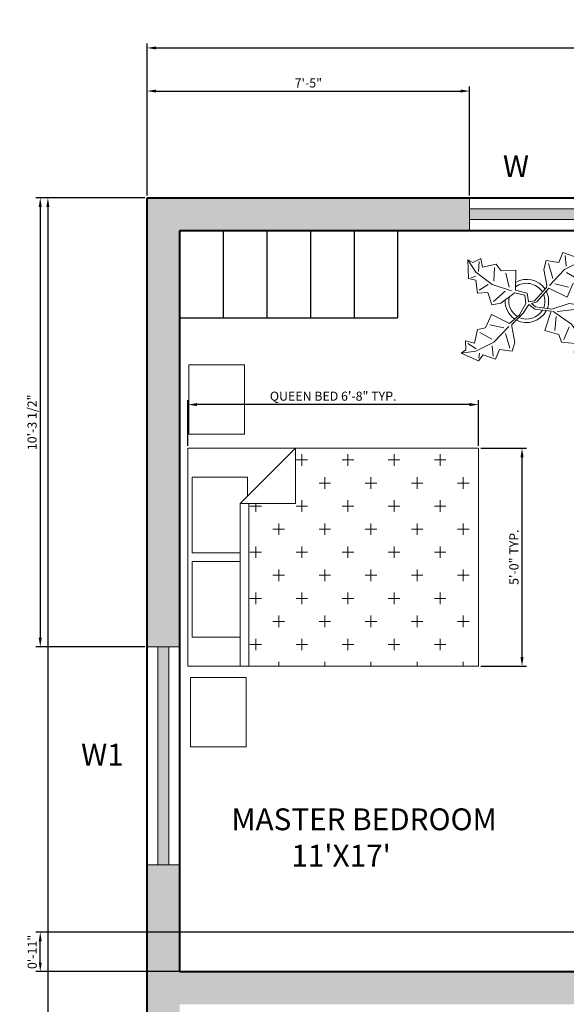
# Model space of a CAD drawing. Units: inches. Extents: x 4432 to 4859, y 8121 to 8698.
# Tile 3 of 4: x 4432 to 4583, y 8410 to 8681. Entities that reach past the tile are written whole.
import ezdxf

# ---------------------------------------------------------------- set-up
doc = ezdxf.new("R2010")
doc.units = ezdxf.units.IN
for name, color, linetype, lineweight in [('A-ANNO-DIMS', 2, 'Continuous', 18), ('A-ANNO-TEXT', 7, 'Continuous', 18), ('A-AREA-IDEN', 4, 'Continuous', 18), ('A-FLOR-CASE', 8, 'Continuous', 25), ('A-FURN', 8, 'Continuous', 18), ('A-FURN-PATT', 8, 'Continuous', 13), ('A-FURN-PLNT', 94, 'Continuous', 13), ('A-GLAZ', 4, 'Continuous', 20), ('A-GLAZ-PATT', 4, 'Continuous', 13), ('A-WALL', 7, 'Continuous', 40)]:
    doc.layers.add(name, color=color, linetype=linetype, lineweight=lineweight)
doc.layers.add('A-WALL-PATT', color=219, linetype='Continuous', lineweight=13, true_color=0x642165)
doc.styles.get("Standard").update_dxf_attribs({"font": 'arial.ttf'})
doc.dimstyles.new('ISO-25', dxfattribs={"dimtxt": 2.5, "dimasz": 2.5, "dimexe": 1.25, "dimexo": 0.625, "dimtad": 1, "dimlunit": 3, "dimtxsty": 'Standard', "dimcen": 2.5, "dimadec": 0, "dimazin": 0, "dimtfac": 1, "dimtmove": 0, "dimatfit": 3, "dimfxl": 1, "dimarcsym": 0})

# ---------------------------------------------------------------- blocks, each defined once
blk = doc.blocks.new('Bed - Queen')
for p, q in [((0, -80.00003), (0, 0)), ((0, 0), (59.99999, 0)), ((59.99999, 0), (59.99999, -80.00003)), ((7.99999, -1.2), (28.79998, -1.2)), ((7.99999, -14.4), (7.99999, -1.2)), ((28.79998, -1.2), (28.79998, -14.4)), ((31.19999, -1.2), (51.99999, -1.2)), ((31.19999, -14.4), (31.19999, -1.2)), ((51.99999, -1.2), (51.99999, -16.4)), ((0, -14.4), (44.8, -14.4)), ((59.99999, -29.6), (44.8, -14.4)), ((44.8, -14.4), (44.8, -29.6)), ((44.8, -16.8), (0, -16.8)), ((51.99999, -16.4), (46.79936, -16.4)), ((44.8, -29.6), (59.99999, -29.6)), ((59.99999, -80.00003), (0, -80.00003))]:
    blk.add_line(p, q)
blk = doc.blocks.new('Plant - Rubber or Philodendron')
for p, q in [((13.3837, 12.301), (14.68, 13.9039)), ((14.68, 13.9039), (19.3848, 11.8146)), ((-16.2005, 11.4774), (-13.9899, 8.1064)), ((-16.2005, 11.4774), (-14.8639, 10.7964)), ((-16.0159, 6.3329), (-16.2005, 11.4774)), ((-14.8639, 10.7964), (-12.6195, 11.8975)), ((-13.3174, 8.325), (-13.0735, 11.0065)), ((-12.6195, 11.8975), (-12.1909, 9.4345)), ((4.6914, 8.8812), (5.3859, 11.2828)), ((5.3859, 11.2828), (8.8871, 10.7908)), ((8.8871, 10.7908), (9.9809, 13.4933)), ((9.9809, 13.4933), (13.3837, 12.301)), ((15.3859, 11.3055), (10.3916, 8.7942)), ((10.5828, 12.6946), (10.8893, 9.7953)), ((14.5816, 13.2037), (14.3848, 11.8033)), ((19.3848, 11.8146), (15.3859, 11.3055)), ((19.3848, 11.8146), (18.1868, 10.9119)), ((18.1868, 10.9119), (18.1925, 8.4119)), ((-12.1909, 9.4345), (-8.3829, 10.3)), ((-8.8369, 9.409), (-9.0894, 5.6095)), ((-8.3829, 10.3), (-7.0549, 8.501)), ((-7.0549, 8.501), (-3.0284, 8.6941)), ((-3.0284, 8.6941), (-3.0709, 3.1041)), ((4.6914, 8.8812), (5.5014, 4.4831)), ((5.9878, 10.4842), (7.1971, 6.3869)), ((10.3916, 8.7942), (6.2847, 4.4028)), ((15.7909, 9.1065), (14.8995, 5.3044)), ((15.2875, 10.6053), (17.5907, 9.2105)), ((18.1925, 8.4119), (15.7909, 9.1065)), ((-14.0069, 5.8704), (-16.0159, 6.3329)), ((-15.3434, 6.5514), (-13.9984, 6.9884)), ((-13.5868, 2.2894), (-14.0069, 5.8704)), ((-13.9899, 8.1064), (-9.5434, 4.7185)), ((-4.8529, 4.012), (-5.7184, 7.82)), ((14.2977, 6.1031), (10.9934, 7.9956)), ((-13.1329, 3.1804), (-10.6614, 4.727)), ((-9.5434, 4.7185), (-4.1917, 2.9888)), ((-9.1318, 0.0195), (-5.9793, 2.9025)), ((-3.0709, 3.1041), (0.0797, 2.3163)), ((2.1141, 0.2298), (5.4346, 3.9146)), ((6.1032, 3.6844), (2.8262, -0.031)), ((5.4346, 3.9146), (5.5014, 4.4831)), ((11.1089, 1.1958), (6.1032, 3.6844)), ((7.7005, 4.8881), (11.5025, 3.9967)), ((12.7005, 4.8994), (11.1089, 1.1958)), ((14.8995, 5.3044), (12.7005, 4.8994)), ((-10.6784, 2.491), (-13.5868, 2.2894)), ((-9.5858, -0.8715), (-10.6784, 2.491)), ((-7.1228, -0.443), (-3.5248, 2.2131)), ((-3.5248, 2.2131), (-3.3011, 2.4355)), ((-3.3011, 2.4355), (-0.5306, 1.7947)), ((-0.5306, 1.7947), (-0.2255, -0.5527)), ((-0.5306, 1.7947), (-0.5306, 1.7947)), ((0.0797, 2.3163), (0.4866, -0.031)), ((0.4866, -0.031), (2.1141, 0.2298)), ((-7.1228, -0.443), (-9.5858, -0.8715)), ((-2.019, -3.6148), (-0.2255, -0.5527)), ((-0.9375, -3.1608), (0.5883, -0.8135)), ((0.5883, -0.8135), (2.2447, -2.0916)), ((2.8262, -0.031), (1.3003, -0.5527)), ((1.3003, -0.5527), (2.4193, -1.4655)), ((2.2447, -2.0916), (6.7108, -2.6626)), ((2.4193, -1.4655), (6.895, -2.1175)), ((4.943, -7.9659), (6.7108, -2.6626)), ((11.6605, -0.5413), (6.895, -2.1175)), ((12.3677, -6.1981), (7.219, -2.6772)), ((8.3544, -2.7453), (13.1973, -2.1704)), ((11.6605, -0.5413), (14.1354, -0.8948)), ((14.1354, -0.8948), (14.1354, -4.4304)), ((-11.3237, -7.2629), (-9.7321, -3.5593)), ((-9.7321, -3.5593), (-4.7264, -6.0479)), ((-2.019, -3.6148), (-4.7264, -6.0479)), ((-4.0579, -6.2781), (-0.9375, -3.1608)), ((8.125, -4.0768), (7.7715, -7.9659)), ((14.1354, -4.4304), (16.9638, -5.1375)), ((16.9638, -5.1375), (16.2567, -8.673)), ((-14.4141, -11.4699), (-13.5228, -7.6679)), ((-13.5228, -7.6679), (-11.3237, -7.2629)), ((-6.3237, -7.2516), (-10.1257, -6.3602)), ((-9.0148, -11.1577), (-4.9047, -6.8122)), ((-4.1246, -6.8466), (-4.0579, -6.2781)), ((-3.3146, -11.2447), (-4.1246, -6.8466)), ((8.8321, -9.0266), (4.943, -7.9659)), ((10.2463, -10.4408), (11.6605, -6.9053)), ((15.5496, -10.7943), (12.3677, -6.1981)), ((16.2567, -5.8446), (13.4283, -6.5517)), ((-16.8157, -10.7754), (-14.4141, -11.4699)), ((-16.8101, -13.2754), (-16.8157, -10.7754)), ((-12.921, -8.4665), (-9.6166, -10.359)), ((-4.611, -12.8477), (-5.8203, -8.7504)), ((9.5392, -11.1479), (8.8321, -9.0266)), ((14.8425, -10.7943), (13.7819, -13.2692)), ((16.6103, -14.6834), (15.5496, -10.7943)), ((17.3174, -9.7337), (15.9032, -9.7337)), ((16.2567, -8.673), (18.0245, -9.7337)), ((18.0245, -9.7337), (16.6103, -14.6834)), ((-18.008, -14.1781), (-16.8101, -13.2754)), ((-13.9107, -12.9688), (-16.2139, -11.574)), ((-14.0091, -13.669), (-9.0148, -11.1577)), ((-9.206, -15.0581), (-9.5126, -12.1588)), ((-7.5103, -13.1543), (-8.6042, -15.8568)), ((-4.0092, -13.6463), (-7.5103, -13.1543)), ((-3.3146, -11.2447), (-4.0092, -13.6463)), ((13.4283, -11.5015), (9.5392, -11.1479)), ((13.0748, -13.9763), (13.4283, -11.5015)), ((-18.008, -14.1781), (-14.0091, -13.669)), ((-13.3032, -16.2674), (-18.008, -14.1781)), ((-12.0069, -14.6645), (-13.3032, -16.2674)), ((-13.2048, -15.5672), (-13.008, -14.1668)), ((-8.6042, -15.8568), (-12.0069, -14.6645)), ((15.5496, -13.6228), (13.0748, -13.9763)), ((16.6103, -14.6834), (15.5496, -13.6228))]:
    blk.add_line(p, q)
for centre, radius, start, end in [((0, 0), 6.1275, 34.37569, 120.1028), ((-0.0601, -0.2075), 5.2461, 33.82192, 124.9414), ((-0.098, 0.1364), 6.1288, 341.2017, 26.09184), ((0.0308, 0.1664), 6, 178.6147, 235.1169), ((0.0308, 0.1664), 5, 168.1647, 238.6725), ((-0.2664, 0.1682), 5.2775, 338.4094, 20.03007), ((-0.0234, 0.3825), 6.1492, 242.5812, 331.2714), ((-0.1102, 0.4886), 5.2883, 247.3711, 327.472)]:
    blk.add_arc(centre, radius, start, end)
blk = doc.blocks.new('*D14')
at = {"layer": 'A-ANNO-DIMS', "color": 0, "lineweight": -2, "transparency": 16777216}
for p, q in [((4467.47, 8632.58), (4467.47, 8674.47)), ((4827.47, 8632.58), (4827.47, 8674.47)), ((4469.97, 8673.22), (4824.97, 8673.22))]:
    blk.add_line(p, q, dxfattribs=at)
at = {"layer": 'A-ANNO-DIMS', "color": 0, "transparency": 16777216}
for points in [[(4469.97, 8673.64), (4469.97, 8672.8), (4467.47, 8673.22)], [(4824.97, 8673.64), (4824.97, 8672.8), (4827.47, 8673.22)]]:
    blk.add_solid(points, dxfattribs=at)
at = {"layer": 'Defpoints', "color": 0, "transparency": 16777216}
for p in [(4827.47, 8673.22), (4467.47, 8631.96), (4827.47, 8631.96)]:
    blk.add_point(p, dxfattribs=at)
at = {"layer": 'A-ANNO-DIMS', "color": 0, "transparency": 16777216, "insert": (4647.47, 8676.91), "char_height": 6, "attachment_point": 5}
blk.add_mtext("30'", dxfattribs=at)
blk = doc.blocks.new('*D15')
at = {"layer": 'A-ANNO-DIMS', "color": 0, "lineweight": -2, "transparency": 16777216}
for p, q in [((4466.84, 8631.96), (4438.93, 8631.96)), ((4440.18, 8629.46), (4440.18, 8154.46)), ((4466.84, 8151.96), (4438.93, 8151.96))]:
    blk.add_line(p, q, dxfattribs=at)
at = {"layer": 'A-ANNO-DIMS', "color": 0, "transparency": 16777216}
for points in [[(4439.77, 8629.46), (4440.6, 8629.46), (4440.18, 8631.96)], [(4439.77, 8154.46), (4440.6, 8154.46), (4440.18, 8151.96)]]:
    blk.add_solid(points, dxfattribs=at)
at = {"layer": 'Defpoints', "color": 0, "transparency": 16777216}
for p in [(4467.47, 8631.96), (4440.18, 8151.96), (4467.47, 8151.96)]:
    blk.add_point(p, dxfattribs=at)
at = {"layer": 'A-ANNO-DIMS', "color": 0, "transparency": 16777216, "insert": (4436.49, 8391.96), "char_height": 6, "attachment_point": 5, "rotation": 90}
blk.add_mtext("40'", dxfattribs=at)
blk = doc.blocks.new('WIN-36IN')
for p, q in [((0, 0), (0, 9)), ((0, 9), (36, 9)), ((36, 9), (36, 0)), ((0, 6), (36, 6)), ((0, 3), (36, 3)), ((36, 0), (0, 0))]:
    blk.add_line(p, q)
blk = doc.blocks.new('WIN-60IN')
for p, q in [((0, 60), (9, 60)), ((0, 60), (0, 0)), ((3, 60), (3, 0)), ((6, 60), (6, 0)), ((9, 0), (9, 60)), ((0, 0), (9, 0)), ((0, 0), (9, 0))]:
    blk.add_line(p, q)
blk = doc.blocks.new('WARDROBE-5BAY-60IN')
for p, q in [((12, 24), (12, 0)), ((24, 24), (24, 0)), ((36, 24), (36, 0)), ((48, 24), (48, 0)), ((60, 24), (60, 0)), ((0, 0), (60, 0))]:
    blk.add_line(p, q)
blk = doc.blocks.new('NIGHTSTAND-RECT')
blk.add_lwpolyline([(0, 19.04), (15.29, 19.04), (15.29, 0), (0, 0)], close=True)
blk = doc.blocks.new('*D35')
at = {"layer": 'A-ANNO-DIMS', "color": 0, "lineweight": -2, "transparency": 16777216}
for p, q in [((4478.73, 8563.67), (4478.73, 8576.29)), ((4558.73, 8563.67), (4558.73, 8576.29)), ((4556.23, 8575.04), (4481.23, 8575.04))]:
    blk.add_line(p, q, dxfattribs=at)
at = {"layer": 'A-ANNO-DIMS', "color": 0, "transparency": 16777216}
for points in [[(4481.23, 8575.46), (4481.23, 8574.63), (4478.73, 8575.04)], [(4556.23, 8575.46), (4556.23, 8574.63), (4558.73, 8575.04)]]:
    blk.add_solid(points, dxfattribs=at)
at = {"layer": 'Defpoints', "color": 0, "transparency": 16777216}
for p in [(4478.73, 8575.04), (4478.73, 8563.04), (4558.73, 8563.04)]:
    blk.add_point(p, dxfattribs=at)
at = {"layer": 'A-ANNO-DIMS', "color": 0, "transparency": 16777216, "insert": (4518.73, 8577.04), "char_height": 2.5, "attachment_point": 5}
blk.add_mtext('QUEEN BED 6\'-8" TYP.', dxfattribs=at)
blk = doc.blocks.new('*D36')
at = {"layer": 'A-ANNO-DIMS', "color": 0, "lineweight": -2, "transparency": 16777216}
for p, q in [((4559.36, 8563.04), (4571.98, 8563.04)), ((4570.73, 8505.54), (4570.73, 8560.54)), ((4559.36, 8503.04), (4571.98, 8503.04))]:
    blk.add_line(p, q, dxfattribs=at)
at = {"layer": 'A-ANNO-DIMS', "color": 0, "transparency": 16777216}
for points in [[(4570.32, 8560.54), (4571.15, 8560.54), (4570.73, 8563.04)], [(4570.32, 8505.54), (4571.15, 8505.54), (4570.73, 8503.04)]]:
    blk.add_solid(points, dxfattribs=at)
at = {"layer": 'Defpoints', "color": 0, "transparency": 16777216}
for p in [(4558.73, 8563.04), (4570.73, 8563.04), (4558.73, 8503.04)]:
    blk.add_point(p, dxfattribs=at)
at = {"layer": 'A-ANNO-DIMS', "color": 0, "transparency": 16777216, "insert": (4568.83, 8533.04), "char_height": 2.5, "attachment_point": 5, "rotation": 90}
blk.add_mtext('5\'-0" TYP.', dxfattribs=at)
blk = doc.blocks.new('*D51')
at = {"layer": 'A-ANNO-DIMS', "color": 0, "lineweight": -2, "transparency": 16777216}
for p, q in [((4467.47, 8632.58), (4467.47, 8662.61)), ((4556.31, 8632.58), (4556.31, 8662.61)), ((4469.97, 8661.36), (4553.81, 8661.36))]:
    blk.add_line(p, q, dxfattribs=at)
at = {"layer": 'A-ANNO-DIMS', "color": 0, "transparency": 16777216}
for points in [[(4469.97, 8661.77), (4469.97, 8660.94), (4467.47, 8661.36)], [(4553.81, 8661.77), (4553.81, 8660.94), (4556.31, 8661.36)]]:
    blk.add_solid(points, dxfattribs=at)
at = {"layer": 'Defpoints', "color": 0, "transparency": 16777216}
for p in [(4556.31, 8661.36), (4467.47, 8631.96), (4556.31, 8631.96)]:
    blk.add_point(p, dxfattribs=at)
at = {"layer": 'A-ANNO-DIMS', "color": 0, "transparency": 16777216, "insert": (4511.89, 8663.25), "char_height": 2.5, "attachment_point": 5}
blk.add_mtext('7\'-5"', dxfattribs=at)
blk = doc.blocks.new('*D63')
at = {"layer": 'A-ANNO-DIMS', "color": 0, "lineweight": -2, "transparency": 16777216}
for p, q in [((4466.84, 8631.96), (4436.82, 8631.96)), ((4438.07, 8629.46), (4438.07, 8510.86)), ((4466.84, 8508.36), (4436.82, 8508.36))]:
    blk.add_line(p, q, dxfattribs=at)
at = {"layer": 'A-ANNO-DIMS', "color": 0, "transparency": 16777216}
for points in [[(4437.65, 8629.46), (4438.48, 8629.46), (4438.07, 8631.96)], [(4437.65, 8510.86), (4438.48, 8510.86), (4438.07, 8508.36)]]:
    blk.add_solid(points, dxfattribs=at)
at = {"layer": 'Defpoints', "color": 0, "transparency": 16777216}
for p in [(4467.47, 8631.96), (4438.07, 8508.36), (4467.47, 8508.36)]:
    blk.add_point(p, dxfattribs=at)
at = {"layer": 'A-ANNO-DIMS', "color": 0, "transparency": 16777216, "insert": (4436.15, 8570.16), "char_height": 2.5, "attachment_point": 5, "rotation": 90}
blk.add_mtext('10\'-3 1/2"', dxfattribs=at)
blk = doc.blocks.new('*D73')
at = {"layer": 'A-ANNO-DIMS', "color": 0, "lineweight": -2, "transparency": 16777216}
for p, q in [((4676.84, 8429.78), (4436.82, 8429.78)), ((4438.07, 8421.46), (4438.07, 8427.28)), ((4685.84, 8418.96), (4436.82, 8418.96))]:
    blk.add_line(p, q, dxfattribs=at)
at = {"layer": 'A-ANNO-DIMS', "color": 0, "transparency": 16777216}
for points in [[(4437.65, 8427.28), (4438.48, 8427.28), (4438.07, 8429.78)], [(4437.65, 8421.46), (4438.48, 8421.46), (4438.07, 8418.96)]]:
    blk.add_solid(points, dxfattribs=at)
at = {"layer": 'Defpoints', "color": 0, "transparency": 16777216}
for p in [(4438.07, 8429.78), (4677.47, 8429.78), (4686.47, 8418.96)]:
    blk.add_point(p, dxfattribs=at)
at = {"layer": 'A-ANNO-DIMS', "color": 0, "transparency": 16777216, "insert": (4436.17, 8424.37), "char_height": 2.5, "attachment_point": 5, "rotation": 90}
blk.add_mtext('0\'-11"', dxfattribs=at)

msp = doc.modelspace()

# ---------------------------------------------------------------- hatches: boundary and pattern name
at = {"layer": 'A-FURN-PATT'}
h = msp.add_hatch(dxfattribs=at)
h.set_pattern_fill('CROSS', color=256)
h.paths.add_polyline_path([(4558.735, 8563.044), (4508.335, 8563.044), (4508.335, 8547.844), (4495.535, 8547.844), (4495.535, 8503.044), (4558.735, 8503.044)])
h.paths.add_polyline_path([(4768.654, 8563.044), (4718.254, 8563.044), (4718.254, 8547.844), (4705.454, 8547.844), (4705.454, 8503.044), (4768.654, 8503.044)])
h.paths.add_polyline_path([(4699.088, 8354.439, 1), (4726.919, 8354.439, 1)])
at = {"layer": 'A-GLAZ-PATT'}
h = msp.add_hatch(color=256, dxfattribs=at)
h.dxf.hatch_style = 1
h.paths.add_polyline_path([(4592.313, 8628.956), (4556.313, 8628.956), (4556.313, 8625.956), (4592.313, 8625.956)])
h.paths.add_polyline_path([(4660.176, 8628.956), (4636.176, 8628.956), (4636.176, 8625.956), (4660.176, 8625.956)])
h.paths.add_polyline_path([(4799.877, 8628.956), (4763.877, 8628.956), (4763.877, 8625.956), (4799.877, 8625.956)])
h.paths.add_polyline_path([(4473.468, 8508.361), (4470.468, 8508.361), (4470.468, 8448.361), (4473.468, 8448.361)])
h.paths.add_polyline_path([(4473.468, 8398.047), (4470.468, 8398.047), (4470.468, 8377.047), (4473.468, 8377.047)])
h.paths.add_polyline_path([(4473.468, 8341.903), (4470.468, 8341.903), (4470.468, 8305.903), (4473.468, 8305.903)])
h.paths.add_polyline_path([(4577.354, 8253.956), (4529.354, 8253.956), (4529.354, 8250.956), (4577.354, 8250.956)])
h.paths.add_polyline_path([(4662.104, 8253.956), (4650.104, 8253.956), (4650.104, 8250.956), (4662.104, 8250.956)])
h.paths.add_polyline_path([(4722.104, 8253.956), (4710.104, 8253.956), (4710.104, 8250.956), (4722.104, 8250.956)])
h.paths.add_polyline_path([(4824.468, 8397.007), (4821.468, 8397.007), (4821.468, 8361.007), (4824.468, 8361.007)])
h.paths.add_polyline_path([(4824.468, 8509.871), (4821.468, 8509.871), (4821.468, 8449.871), (4824.468, 8449.871)])
at = {"layer": 'A-WALL-PATT'}
h = msp.add_hatch(color=256, dxfattribs=at)
h.dxf.hatch_style = 1
h.paths.add_polyline_path([(4556.313, 8631.956), (4467.468, 8631.956), (4467.468, 8508.361), (4476.468, 8508.361), (4476.468, 8622.956), (4556.313, 8622.956)])
h.paths.add_polyline_path([(4636.176, 8631.956), (4592.313, 8631.956), (4592.313, 8622.956), (4608.468, 8622.956), (4608.468, 8546.941), (4617.468, 8546.941), (4617.468, 8622.956), (4636.176, 8622.956)])
h.paths.add_polyline_path([(4763.877, 8631.956), (4660.176, 8631.956), (4660.176, 8622.956), (4677.468, 8622.956), (4677.468, 8502.956), (4617.468, 8502.956), (4617.468, 8524.355), (4608.468, 8524.355), (4608.468, 8459.776), (4615.468, 8459.776, -0.0172363), (4617.468, 8459.776), (4617.468, 8493.956), (4677.468, 8493.956), (4677.468, 8459.776, -0.0172363), (4679.468, 8459.776), (4686.468, 8459.776), (4686.468, 8622.956), (4763.877, 8622.956)])
h.paths.add_polyline_path([(4827.468, 8631.956), (4799.877, 8631.956), (4799.877, 8622.956), (4818.468, 8622.956), (4818.468, 8509.871), (4827.468, 8509.871)])
h.paths.add_polyline_path([(4617.468, 8429.776), (4608.468, 8429.776), (4608.468, 8418.956), (4476.468, 8418.956), (4476.468, 8448.361), (4467.468, 8448.361), (4467.468, 8398.047), (4476.468, 8398.047), (4476.468, 8409.956), (4608.468, 8409.956), (4608.468, 8397.41), (4612.05, 8397.41, -0.0497121), (4617.468, 8397.41)])
h.paths.add_polyline_path([(4827.468, 8449.871), (4818.468, 8449.871), (4818.468, 8418.956), (4686.468, 8418.956), (4686.468, 8429.776), (4677.468, 8429.776), (4677.468, 8409.956), (4818.468, 8409.956), (4818.468, 8397.007), (4827.468, 8397.007)])
h.paths.add_polyline_path([(4617.468, 8369.235), (4608.468, 8369.235), (4608.468, 8361.956), (4476.468, 8361.956), (4476.468, 8377.047), (4467.468, 8377.047), (4467.468, 8341.903), (4476.468, 8341.903), (4476.468, 8352.956), (4617.468, 8352.956)])
h.paths.add_polyline_path([(4529.354, 8256.956), (4476.468, 8256.956), (4476.468, 8305.903), (4467.468, 8305.903), (4467.468, 8151.956), (4650.104, 8151.956), (4650.104, 8157.956), (4471.968, 8157.956), (4471.968, 8169.956), (4599.396, 8169.956), (4599.396, 8174.456), (4476.468, 8174.456), (4476.468, 8247.956), (4529.354, 8247.956)])
h.paths.add_polyline_path([(4650.104, 8256.956), (4617.468, 8256.956), (4617.468, 8304.956), (4608.468, 8304.956), (4608.468, 8256.956), (4577.354, 8256.956), (4577.354, 8247.956), (4650.104, 8247.956)], flags=17)
h.paths.add_polyline_path([(4827.468, 8361.007), (4818.468, 8361.007), (4818.468, 8333.456), (4807.435, 8333.456, -0.0172363), (4807.435, 8331.456), (4807.435, 8328.956), (4818.468, 8328.956), (4818.468, 8256.956), (4770.468, 8256.956), (4770.468, 8328.956), (4777.435, 8328.956), (4777.435, 8333.456), (4765.968, 8333.456), (4765.968, 8256.956), (4722.104, 8256.956), (4722.104, 8247.956), (4821.468, 8247.956), (4821.468, 8157.956), (4765.968, 8157.956), (4765.968, 8151.956), (4827.468, 8151.956)])
h.paths.add_polyline_path([(4765.968, 8154.956), (4650.104, 8154.956), (4650.104, 8151.956), (4765.968, 8151.956)])

# ---------------------------------------------------------------- linework, layer by layer
at = {"layer": 'A-FLOR-CASE'}
msp.add_line((4476.468, 8622.956), (4476.468, 8598.956), dxfattribs=at)
at = {"layer": 'A-WALL'}
for p, q in [((4467.468, 8631.956), (4827.468, 8631.956)), ((4467.468, 8151.956), (4467.468, 8631.956)), ((4476.468, 8622.956), (4608.468, 8622.956)), ((4476.468, 8418.956), (4476.468, 8622.956)), ((4476.468, 8418.956), (4608.468, 8418.956))]:
    msp.add_line(p, q, dxfattribs=at)

# ---------------------------------------------------------------- block references
at = {"layer": 'A-FLOR-CASE'}
msp.add_blockref('WARDROBE-5BAY-60IN', (4476.468, 8598.956), dxfattribs=at)
at = {"layer": 'A-FURN'}
for p in [(4479.017, 8566.907), (4479.486, 8480.857)]:
    msp.add_blockref('NIGHTSTAND-RECT', p, dxfattribs=at)
at = {"layer": 'A-FURN', "rotation": 90}
msp.add_blockref('Bed - Queen', (4478.735, 8503.044), dxfattribs=at)
at = {"layer": 'A-FURN-PLNT'}
msp.add_blockref('Plant - Rubber or Philodendron', (4572.026, 8603.394), dxfattribs=at)
at = {"layer": 'A-GLAZ'}
msp.add_blockref('WIN-36IN', (4556.313, 8622.956), dxfattribs=at)
at = {"layer": 'A-GLAZ', "rotation": 180}
msp.add_blockref('WIN-60IN', (4476.468, 8508.361), dxfattribs=at)

# ---------------------------------------------------------------- texts
at = {"layer": 'A-ANNO-TEXT', "char_height": 6, "attachment_point": 1}
for s, insert in [('W  ', (4565.471, 8643.674)), ('W1', (4449.325, 8481.693))]:
    msp.add_mtext_dynamic_manual_height_columns(s, width=117.51606, gutter_width=12.5, heights=[0], dxfattribs=dict(at, insert=insert))
at = {"layer": 'A-AREA-IDEN', "insert": (4488.867, 8463.885), "char_height": 6, "attachment_point": 1}
msp.add_mtext_dynamic_manual_height_columns(" {MASTER BEDROOM\\P          11'X17'}", width=117.51606, gutter_width=12.5, heights=[0], dxfattribs=at)

# ---------------------------------------------------------------- dimensions: what is measured, and where the dimension line sits
at = {"layer": 'A-ANNO-DIMS'}
for base, p2, override, picture, middle in [((4827.468, 8673.218), (4827.468, 8631.956), {"dimtxt": 6, "dimclrd": 0, "dimclre": 0, "dimclrt": 0}, '*D14', (4647.468, 8676.909)), ((4556.313, 8661.356), (4556.313, 8631.956), {"dimdec": 1, "dimlfac": 1, "dimrnd": 0, "dimzin": 1, "dimdsep": 46, "dimlunit": 4, "dimfrac": 2}, '*D51', (4511.89, 8663.253))]:
    dim = msp.add_linear_dim(base=base, p1=(4467.468, 8631.956), p2=p2, dimstyle='ISO-25', override=override, dxfattribs=at)
    dim.commit()
    dim.dimension.update_dxf_attribs({"geometry": picture, "text_midpoint": middle})
for base, p1, p2, override, picture, middle in [((4440.183, 8151.956), (4467.468, 8631.956), (4467.468, 8151.956), {"dimtxt": 6, "dimclrd": 0, "dimclre": 0, "dimclrt": 0}, '*D15', (4436.494, 8391.956)), ((4438.068, 8508.361), (4467.468, 8631.956), (4467.468, 8508.361), {"dimdec": 1, "dimlfac": 1, "dimrnd": 0, "dimzin": 1, "dimdsep": 46, "dimlunit": 4, "dimfrac": 2}, '*D63', (4436.149, 8570.159)), ((4438.068, 8429.776), (4686.468, 8418.956), (4677.468, 8429.776), {"dimdec": 1, "dimlfac": 1, "dimrnd": 0, "dimzin": 1, "dimdsep": 46, "dimlunit": 4, "dimfrac": 2}, '*D73', (4436.166, 8424.366))]:
    dim = msp.add_linear_dim(base=base, p1=p1, p2=p2, angle=90, dimstyle='ISO-25', override=override, dxfattribs=at)
    dim.commit()
    dim.dimension.update_dxf_attribs({"geometry": picture, "text_midpoint": middle})
for base, p1, p2, angle, text, picture, middle in [((4478.735, 8575.044), (4558.735, 8563.044), (4478.735, 8563.044), 180, 'QUEEN BED <> TYP.', '*D35', (4518.735, 8577.039)), ((4570.735, 8563.044), (4558.735, 8503.044), (4558.735, 8563.044), 90, '<> TYP.', '*D36', (4568.833, 8533.044))]:
    dim = msp.add_linear_dim(base=base, p1=p1, p2=p2, angle=angle, text=text, dimstyle='ISO-25', override={"dimdec": 1, "dimlfac": 1, "dimrnd": 0, "dimzin": 1, "dimdsep": 46, "dimlunit": 4, "dimfrac": 2}, dxfattribs=at)
    dim.commit()
    dim.dimension.update_dxf_attribs({"geometry": picture, "text_midpoint": middle})

doc.saveas('drawing.dxf')
